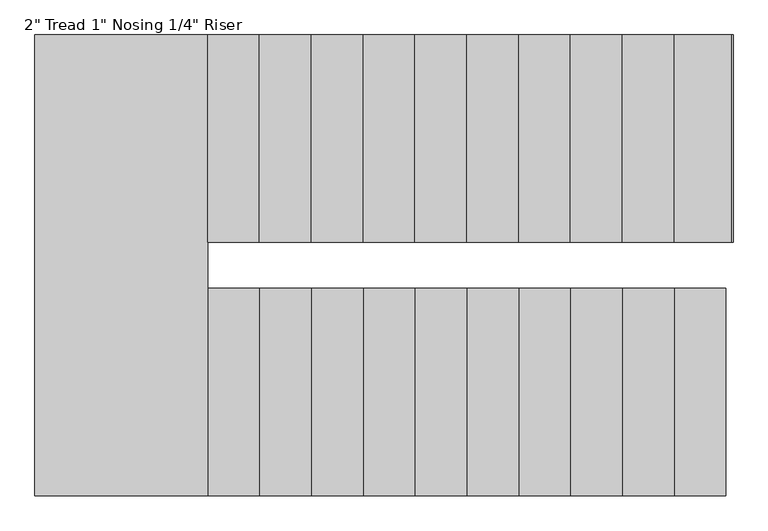
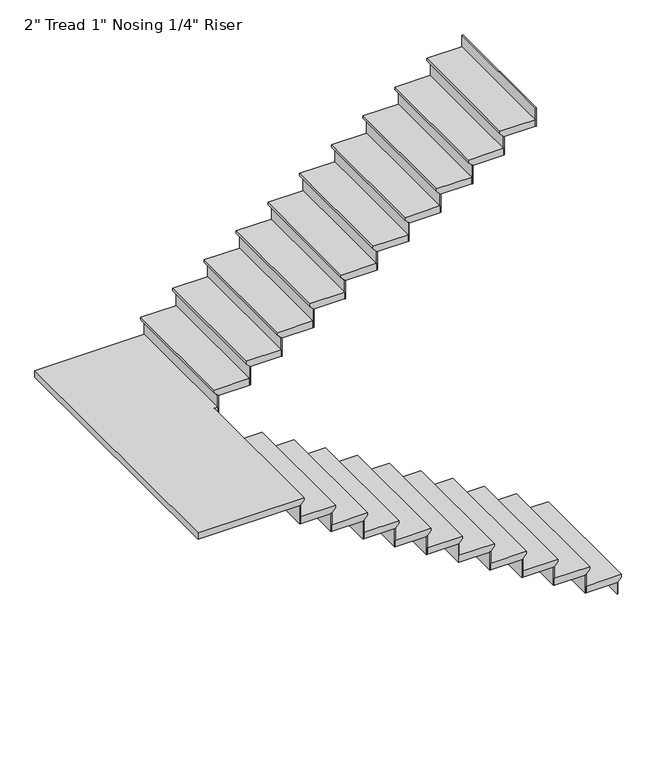
"""IFC4 building model written with IfcOpenShell, lengths in millimetres: stair flight geometry."""

from ifc_helpers import new_model, si_unit, origin, place, context, project, spatial, faceted_brep, source, transform, mapped, element, save


def stair_flight_0d4d62c4(model_context):
    return source(origin(), model_context, "Body", "Brep", [
        faceted_brep([(-2080.8410855, 332.1803617, 16121.4954545), (-2080.8410855, 332.1803617, 16140.5454545), (-2080.8410855, -582.2196383, 16140.5454545), (-2080.8410855, -582.2196383, 16121.4954545), (-2106.2410855, 332.1803617, 16096.0954545), (-2106.2410855, -582.2196383, 16096.0954545), (-2334.8410855, 332.1803617, 16140.5454545), (-2334.8410855, -582.2196383, 16140.5454545), (-2106.2410855, -582.2196383, 16089.7454545), (-2334.8410855, -582.2196383, 16089.7454545), (-2334.8410855, 332.1803617, 16089.7454545), (-2106.2410855, 332.1803617, 16089.7454545)], [[[0, 1, 2, 3]], [[4, 0, 3, 5]], [[2, 1, 6, 7]], [[8, 9, 10, 11]], [[2, 7, 9, 8, 5, 3]], [[8, 11, 4, 5]], [[6, 1, 0, 4, 11, 10]], [[7, 6, 10, 9]]]),
        faceted_brep([(-2106.2410855, 332.1803617, 16089.7454545), (-2106.2410855, 332.1803617, 16002.0), (-2112.5910855, 332.1803617, 16002.0), (-2112.5910855, 332.1803617, 16089.7454545), (-2106.2410855, -582.2196383, 16089.7454545), (-2112.5910855, -582.2196383, 16089.7454545), (-2112.5910855, -582.2196383, 16002.0), (-2106.2410855, -582.2196383, 16002.0)], [[[0, 1, 2, 3]], [[4, 5, 6, 7]], [[1, 0, 4, 7]], [[2, 1, 7, 6]], [[3, 2, 6, 5]], [[0, 3, 5, 4]]]),
        faceted_brep([(-2334.8410855, 332.1803617, 16228.2909091), (-2334.8410855, 332.1803617, 16089.7454545), (-2341.1910855, 332.1803617, 16089.7454545), (-2341.1910855, 332.1803617, 16228.2909091), (-2334.8410855, -582.2196383, 16228.2909091), (-2341.1910855, -582.2196383, 16228.2909091), (-2341.1910855, -582.2196383, 16089.7454545), (-2334.8410855, -582.2196383, 16089.7454545)], [[[0, 1, 2, 3]], [[4, 5, 6, 7]], [[1, 0, 4, 7]], [[2, 1, 7, 6]], [[3, 2, 6, 5]], [[0, 3, 5, 4]]]),
        faceted_brep([(-2309.4410855, -582.2196383, 16279.0909091), (-2309.4410855, 332.1803617, 16279.0909091), (-2563.4410855, 332.1803617, 16279.0909091), (-2563.4410855, -582.2196383, 16279.0909091), (-2334.8410855, -582.2196383, 16228.2909091), (-2563.4410855, -582.2196383, 16228.2909091), (-2563.4410855, 332.1803617, 16228.2909091), (-2334.8410855, 332.1803617, 16228.2909091), (-2334.8410855, -582.2196383, 16234.6409091), (-2309.4410855, -582.2196383, 16260.0409091), (-2334.8410855, 332.1803617, 16234.6409091), (-2309.4410855, 332.1803617, 16260.0409091)], [[[0, 1, 2, 3]], [[4, 5, 6, 7]], [[0, 3, 5, 4, 8, 9]], [[4, 7, 10, 8]], [[2, 1, 11, 10, 7, 6]], [[3, 2, 6, 5]], [[11, 1, 0, 9]], [[10, 11, 9, 8]]]),
        faceted_brep([(-2563.4410855, 332.1803617, 16366.8363636), (-2563.4410855, 332.1803617, 16228.2909091), (-2569.7910855, 332.1803617, 16228.2909091), (-2569.7910855, 332.1803617, 16366.8363636), (-2563.4410855, -582.2196383, 16366.8363636), (-2569.7910855, -582.2196383, 16366.8363636), (-2569.7910855, -582.2196383, 16228.2909091), (-2563.4410855, -582.2196383, 16228.2909091)], [[[0, 1, 2, 3]], [[4, 5, 6, 7]], [[1, 0, 4, 7]], [[2, 1, 7, 6]], [[3, 2, 6, 5]], [[0, 3, 5, 4]]]),
        faceted_brep([(-2538.0410855, -582.2196383, 16417.6363636), (-2538.0410855, 332.1803617, 16417.6363636), (-2792.0410855, 332.1803617, 16417.6363636), (-2792.0410855, -582.2196383, 16417.6363636), (-2563.4410855, -582.2196383, 16366.8363636), (-2792.0410855, -582.2196383, 16366.8363636), (-2792.0410855, 332.1803617, 16366.8363636), (-2563.4410855, 332.1803617, 16366.8363636), (-2563.4410855, -582.2196383, 16373.1863636), (-2538.0410855, -582.2196383, 16398.5863636), (-2563.4410855, 332.1803617, 16373.1863636), (-2538.0410855, 332.1803617, 16398.5863636)], [[[0, 1, 2, 3]], [[4, 5, 6, 7]], [[0, 3, 5, 4, 8, 9]], [[4, 7, 10, 8]], [[2, 1, 11, 10, 7, 6]], [[3, 2, 6, 5]], [[11, 1, 0, 9]], [[10, 11, 9, 8]]]),
        faceted_brep([(-2792.0410855, 332.1803617, 16505.3818182), (-2792.0410855, 332.1803617, 16366.8363636), (-2798.3910855, 332.1803617, 16366.8363636), (-2798.3910855, 332.1803617, 16505.3818182), (-2792.0410855, -582.2196383, 16505.3818182), (-2798.3910855, -582.2196383, 16505.3818182), (-2798.3910855, -582.2196383, 16366.8363636), (-2792.0410855, -582.2196383, 16366.8363636)], [[[0, 1, 2, 3]], [[4, 5, 6, 7]], [[1, 0, 4, 7]], [[2, 1, 7, 6]], [[3, 2, 6, 5]], [[0, 3, 5, 4]]]),
        faceted_brep([(-2766.6410855, -582.2196383, 16556.1818182), (-2766.6410855, 332.1803617, 16556.1818182), (-3020.6410855, 332.1803617, 16556.1818182), (-3020.6410855, -582.2196383, 16556.1818182), (-2792.0410855, -582.2196383, 16505.3818182), (-3020.6410855, -582.2196383, 16505.3818182), (-3020.6410855, 332.1803617, 16505.3818182), (-2792.0410855, 332.1803617, 16505.3818182), (-2792.0410855, -582.2196383, 16511.7318182), (-2766.6410855, -582.2196383, 16537.1318182), (-2792.0410855, 332.1803617, 16511.7318182), (-2766.6410855, 332.1803617, 16537.1318182)], [[[0, 1, 2, 3]], [[4, 5, 6, 7]], [[0, 3, 5, 4, 8, 9]], [[4, 7, 10, 8]], [[2, 1, 11, 10, 7, 6]], [[3, 2, 6, 5]], [[11, 1, 0, 9]], [[10, 11, 9, 8]]]),
        faceted_brep([(-3020.6410855, 332.1803617, 16643.9272727), (-3020.6410855, 332.1803617, 16505.3818182), (-3026.9910855, 332.1803617, 16505.3818182), (-3026.9910855, 332.1803617, 16643.9272727), (-3020.6410855, -582.2196383, 16643.9272727), (-3026.9910855, -582.2196383, 16643.9272727), (-3026.9910855, -582.2196383, 16505.3818182), (-3020.6410855, -582.2196383, 16505.3818182)], [[[0, 1, 2, 3]], [[4, 5, 6, 7]], [[1, 0, 4, 7]], [[2, 1, 7, 6]], [[3, 2, 6, 5]], [[0, 3, 5, 4]]]),
        faceted_brep([(-2995.2410855, -582.2196383, 16694.7272727), (-2995.2410855, 332.1803617, 16694.7272727), (-3249.2410855, 332.1803617, 16694.7272727), (-3249.2410855, -582.2196383, 16694.7272727), (-3020.6410855, -582.2196383, 16643.9272727), (-3249.2410855, -582.2196383, 16643.9272727), (-3249.2410855, 332.1803617, 16643.9272727), (-3020.6410855, 332.1803617, 16643.9272727), (-3020.6410855, -582.2196383, 16650.2772727), (-2995.2410855, -582.2196383, 16675.6772727), (-3020.6410855, 332.1803617, 16650.2772727), (-2995.2410855, 332.1803617, 16675.6772727)], [[[0, 1, 2, 3]], [[4, 5, 6, 7]], [[0, 3, 5, 4, 8, 9]], [[4, 7, 10, 8]], [[2, 1, 11, 10, 7, 6]], [[3, 2, 6, 5]], [[11, 1, 0, 9]], [[10, 11, 9, 8]]]),
        faceted_brep([(-3249.2410855, 332.1803617, 16782.4727273), (-3249.2410855, 332.1803617, 16643.9272727), (-3255.5910855, 332.1803617, 16643.9272727), (-3255.5910855, 332.1803617, 16782.4727273), (-3249.2410855, -582.2196383, 16782.4727273), (-3255.5910855, -582.2196383, 16782.4727273), (-3255.5910855, -582.2196383, 16643.9272727), (-3249.2410855, -582.2196383, 16643.9272727)], [[[0, 1, 2, 3]], [[4, 5, 6, 7]], [[1, 0, 4, 7]], [[2, 1, 7, 6]], [[3, 2, 6, 5]], [[0, 3, 5, 4]]]),
        faceted_brep([(-3223.8410855, -582.2196383, 16833.2727273), (-3223.8410855, 332.1803617, 16833.2727273), (-3477.8410855, 332.1803617, 16833.2727273), (-3477.8410855, -582.2196383, 16833.2727273), (-3249.2410855, -582.2196383, 16782.4727273), (-3477.8410855, -582.2196383, 16782.4727273), (-3477.8410855, 332.1803617, 16782.4727273), (-3249.2410855, 332.1803617, 16782.4727273), (-3249.2410855, -582.2196383, 16788.8227273), (-3223.8410855, -582.2196383, 16814.2227273), (-3249.2410855, 332.1803617, 16788.8227273), (-3223.8410855, 332.1803617, 16814.2227273)], [[[0, 1, 2, 3]], [[4, 5, 6, 7]], [[0, 3, 5, 4, 8, 9]], [[4, 7, 10, 8]], [[2, 1, 11, 10, 7, 6]], [[3, 2, 6, 5]], [[11, 1, 0, 9]], [[10, 11, 9, 8]]]),
        faceted_brep([(-3477.8410855, 332.1803617, 16921.0181818), (-3477.8410855, 332.1803617, 16782.4727273), (-3484.1910855, 332.1803617, 16782.4727273), (-3484.1910855, 332.1803617, 16921.0181818), (-3477.8410855, -582.2196383, 16921.0181818), (-3484.1910855, -582.2196383, 16921.0181818), (-3484.1910855, -582.2196383, 16782.4727273), (-3477.8410855, -582.2196383, 16782.4727273)], [[[0, 1, 2, 3]], [[4, 5, 6, 7]], [[1, 0, 4, 7]], [[2, 1, 7, 6]], [[3, 2, 6, 5]], [[0, 3, 5, 4]]]),
        faceted_brep([(-3452.4410855, -582.2196383, 16971.8181818), (-3452.4410855, 332.1803617, 16971.8181818), (-3706.4410855, 332.1803617, 16971.8181818), (-3706.4410855, -582.2196383, 16971.8181818), (-3477.8410855, -582.2196383, 16921.0181818), (-3706.4410855, -582.2196383, 16921.0181818), (-3706.4410855, 332.1803617, 16921.0181818), (-3477.8410855, 332.1803617, 16921.0181818), (-3477.8410855, -582.2196383, 16927.3681818), (-3452.4410855, -582.2196383, 16952.7681818), (-3477.8410855, 332.1803617, 16927.3681818), (-3452.4410855, 332.1803617, 16952.7681818)], [[[0, 1, 2, 3]], [[4, 5, 6, 7]], [[0, 3, 5, 4, 8, 9]], [[4, 7, 10, 8]], [[2, 1, 11, 10, 7, 6]], [[3, 2, 6, 5]], [[11, 1, 0, 9]], [[10, 11, 9, 8]]]),
        faceted_brep([(-3706.4410855, 332.1803617, 17059.5636364), (-3706.4410855, 332.1803617, 16921.0181818), (-3712.7910855, 332.1803617, 16921.0181818), (-3712.7910855, 332.1803617, 17059.5636364), (-3706.4410855, -582.2196383, 17059.5636364), (-3712.7910855, -582.2196383, 17059.5636364), (-3712.7910855, -582.2196383, 16921.0181818), (-3706.4410855, -582.2196383, 16921.0181818)], [[[0, 1, 2, 3]], [[4, 5, 6, 7]], [[1, 0, 4, 7]], [[2, 1, 7, 6]], [[3, 2, 6, 5]], [[0, 3, 5, 4]]]),
        faceted_brep([(-3681.0410855, -582.2196383, 17110.3636364), (-3681.0410855, 332.1803617, 17110.3636364), (-3935.0410855, 332.1803617, 17110.3636364), (-3935.0410855, -582.2196383, 17110.3636364), (-3706.4410855, -582.2196383, 17059.5636364), (-3935.0410855, -582.2196383, 17059.5636364), (-3935.0410855, 332.1803617, 17059.5636364), (-3706.4410855, 332.1803617, 17059.5636364), (-3706.4410855, -582.2196383, 17065.9136364), (-3681.0410855, -582.2196383, 17091.3136364), (-3706.4410855, 332.1803617, 17065.9136364), (-3681.0410855, 332.1803617, 17091.3136364)], [[[0, 1, 2, 3]], [[4, 5, 6, 7]], [[0, 3, 5, 4, 8, 9]], [[4, 7, 10, 8]], [[2, 1, 11, 10, 7, 6]], [[3, 2, 6, 5]], [[11, 1, 0, 9]], [[10, 11, 9, 8]]]),
        faceted_brep([(-3935.0410855, 332.1803617, 17198.1090909), (-3935.0410855, 332.1803617, 17059.5636364), (-3941.3910855, 332.1803617, 17059.5636364), (-3941.3910855, 332.1803617, 17198.1090909), (-3935.0410855, -582.2196383, 17198.1090909), (-3941.3910855, -582.2196383, 17198.1090909), (-3941.3910855, -582.2196383, 17059.5636364), (-3935.0410855, -582.2196383, 17059.5636364)], [[[0, 1, 2, 3]], [[4, 5, 6, 7]], [[1, 0, 4, 7]], [[2, 1, 7, 6]], [[3, 2, 6, 5]], [[0, 3, 5, 4]]]),
        faceted_brep([(-3909.6410855, -582.2196383, 17248.9090909), (-3909.6410855, 332.1803617, 17248.9090909), (-4163.6410855, 332.1803617, 17248.9090909), (-4163.6410855, -582.2196383, 17248.9090909), (-3935.0410855, -582.2196383, 17198.1090909), (-4163.6410855, -582.2196383, 17198.1090909), (-4163.6410855, 332.1803617, 17198.1090909), (-3935.0410855, 332.1803617, 17198.1090909), (-3935.0410855, -582.2196383, 17204.4590909), (-3909.6410855, -582.2196383, 17229.8590909), (-3935.0410855, 332.1803617, 17204.4590909), (-3909.6410855, 332.1803617, 17229.8590909)], [[[0, 1, 2, 3]], [[4, 5, 6, 7]], [[0, 3, 5, 4, 8, 9]], [[4, 7, 10, 8]], [[2, 1, 11, 10, 7, 6]], [[3, 2, 6, 5]], [[11, 1, 0, 9]], [[10, 11, 9, 8]]]),
        faceted_brep([(-4163.6410855, 332.1803617, 17336.6545455), (-4163.6410855, 332.1803617, 17198.1090909), (-4169.9910855, 332.1803617, 17198.1090909), (-4169.9910855, 332.1803617, 17336.6545455), (-4163.6410855, -582.2196383, 17336.6545455), (-4169.9910855, -582.2196383, 17336.6545455), (-4169.9910855, -582.2196383, 17198.1090909), (-4163.6410855, -582.2196383, 17198.1090909)], [[[0, 1, 2, 3]], [[4, 5, 6, 7]], [[1, 0, 4, 7]], [[2, 1, 7, 6]], [[3, 2, 6, 5]], [[0, 3, 5, 4]]]),
        faceted_brep([(-4138.2410855, -582.2196383, 17387.4545455), (-4138.2410855, 332.1803617, 17387.4545455), (-4392.2410855, 332.1803617, 17387.4545455), (-4392.2410855, -582.2196383, 17387.4545455), (-4163.6410855, -582.2196383, 17336.6545455), (-4392.2410855, -582.2196383, 17336.6545455), (-4392.2410855, 332.1803617, 17336.6545455), (-4163.6410855, 332.1803617, 17336.6545455), (-4163.6410855, -582.2196383, 17343.0045455), (-4138.2410855, -582.2196383, 17368.4045455), (-4163.6410855, 332.1803617, 17343.0045455), (-4138.2410855, 332.1803617, 17368.4045455)], [[[0, 1, 2, 3]], [[4, 5, 6, 7]], [[0, 3, 5, 4, 8, 9]], [[4, 7, 10, 8]], [[2, 1, 11, 10, 7, 6]], [[3, 2, 6, 5]], [[11, 1, 0, 9]], [[10, 11, 9, 8]]]),
        faceted_brep([(-4392.2410855, 332.1803617, 17475.2), (-4392.2410855, 332.1803617, 17336.6545455), (-4398.5910855, 332.1803617, 17336.6545455), (-4398.5910855, 332.1803617, 17475.2), (-4392.2410855, -582.2196383, 17475.2), (-4398.5910855, -582.2196383, 17475.2), (-4398.5910855, -582.2196383, 17336.6545455), (-4392.2410855, -582.2196383, 17336.6545455)], [[[0, 1, 2, 3]], [[4, 5, 6, 7]], [[1, 0, 4, 7]], [[2, 1, 7, 6]], [[3, 2, 6, 5]], [[0, 3, 5, 4]]]),
        faceted_brep([(-4341.4410855, 1449.7803617, 17526.0), (-5128.8410855, 1449.7803617, 17526.0), (-5128.8410855, -582.2196383, 17526.0), (-4366.8410855, -582.2196383, 17526.0), (-4366.8410855, 535.3803617, 17526.0), (-4341.4410855, 535.3803617, 17526.0), (-5128.8410855, 1449.7803617, 17475.2), (-4341.4410855, 1449.7803617, 17475.2), (-4341.4410855, 535.3803617, 17475.2), (-4366.8410855, 535.3803617, 17475.2), (-4366.8410855, 332.1803617, 17475.2), (-4392.2410855, 332.1803617, 17475.2), (-4392.2410855, -582.2196383, 17475.2), (-5128.8410855, -582.2196383, 17475.2), (-4392.2410855, -582.2196383, 17481.55), (-4366.8410855, -582.2196383, 17506.95), (-4392.2410855, 332.1803617, 17481.55), (-4366.8410855, 332.1803617, 17506.95)], [[[0, 1, 2, 3, 4, 5]], [[6, 7, 8, 9, 10, 11, 12, 13]], [[1, 0, 7, 6]], [[2, 1, 6, 13]], [[3, 2, 13, 12, 14, 15]], [[12, 11, 16, 14]], [[11, 10, 17, 16]], [[4, 3, 15, 17, 10, 9]], [[5, 4, 9, 8]], [[0, 5, 8, 7]], [[15, 14, 16, 17]]]),
        faceted_brep([(-4341.4410855, 535.3803617, 17613.7454545), (-4341.4410855, 535.3803617, 17475.2), (-4335.0910855, 535.3803617, 17475.2), (-4335.0910855, 535.3803617, 17613.7454545), (-4341.4410855, 1449.7803617, 17613.7454545), (-4335.0910855, 1449.7803617, 17613.7454545), (-4335.0910855, 1449.7803617, 17475.2), (-4341.4410855, 1449.7803617, 17475.2)], [[[0, 1, 2, 3]], [[4, 5, 6, 7]], [[1, 0, 4, 7]], [[2, 1, 7, 6]], [[3, 2, 6, 5]], [[0, 3, 5, 4]]]),
        faceted_brep([(-4366.8410855, 1449.7803617, 17664.5454545), (-4366.8410855, 535.3803617, 17664.5454545), (-4112.8410855, 535.3803617, 17664.5454545), (-4112.8410855, 1449.7803617, 17664.5454545), (-4341.4410855, 1449.7803617, 17613.7454545), (-4112.8410855, 1449.7803617, 17613.7454545), (-4112.8410855, 535.3803617, 17613.7454545), (-4341.4410855, 535.3803617, 17613.7454545), (-4341.4410855, 1449.7803617, 17620.0954545), (-4366.8410855, 1449.7803617, 17645.4954545), (-4341.4410855, 535.3803617, 17620.0954545), (-4366.8410855, 535.3803617, 17645.4954545)], [[[0, 1, 2, 3]], [[4, 5, 6, 7]], [[0, 3, 5, 4, 8, 9]], [[4, 7, 10, 8]], [[2, 1, 11, 10, 7, 6]], [[3, 2, 6, 5]], [[11, 1, 0, 9]], [[10, 11, 9, 8]]]),
        faceted_brep([(-4112.8410855, 535.3803617, 17752.2909091), (-4112.8410855, 535.3803617, 17613.7454545), (-4106.4910855, 535.3803617, 17613.7454545), (-4106.4910855, 535.3803617, 17752.2909091), (-4112.8410855, 1449.7803617, 17752.2909091), (-4106.4910855, 1449.7803617, 17752.2909091), (-4106.4910855, 1449.7803617, 17613.7454545), (-4112.8410855, 1449.7803617, 17613.7454545)], [[[0, 1, 2, 3]], [[4, 5, 6, 7]], [[1, 0, 4, 7]], [[2, 1, 7, 6]], [[3, 2, 6, 5]], [[0, 3, 5, 4]]]),
        faceted_brep([(-4138.2410855, 1449.7803617, 17803.0909091), (-4138.2410855, 535.3803617, 17803.0909091), (-3884.2410855, 535.3803617, 17803.0909091), (-3884.2410855, 1449.7803617, 17803.0909091), (-4112.8410855, 1449.7803617, 17752.2909091), (-3884.2410855, 1449.7803617, 17752.2909091), (-3884.2410855, 535.3803617, 17752.2909091), (-4112.8410855, 535.3803617, 17752.2909091), (-4112.8410855, 1449.7803617, 17758.6409091), (-4138.2410855, 1449.7803617, 17784.0409091), (-4112.8410855, 535.3803617, 17758.6409091), (-4138.2410855, 535.3803617, 17784.0409091)], [[[0, 1, 2, 3]], [[4, 5, 6, 7]], [[0, 3, 5, 4, 8, 9]], [[4, 7, 10, 8]], [[2, 1, 11, 10, 7, 6]], [[3, 2, 6, 5]], [[11, 1, 0, 9]], [[10, 11, 9, 8]]]),
        faceted_brep([(-3884.2410855, 535.3803617, 17890.8363636), (-3884.2410855, 535.3803617, 17752.2909091), (-3877.8910855, 535.3803617, 17752.2909091), (-3877.8910855, 535.3803617, 17890.8363636), (-3884.2410855, 1449.7803617, 17890.8363636), (-3877.8910855, 1449.7803617, 17890.8363636), (-3877.8910855, 1449.7803617, 17752.2909091), (-3884.2410855, 1449.7803617, 17752.2909091)], [[[0, 1, 2, 3]], [[4, 5, 6, 7]], [[1, 0, 4, 7]], [[2, 1, 7, 6]], [[3, 2, 6, 5]], [[0, 3, 5, 4]]]),
        faceted_brep([(-3909.6410855, 1449.7803617, 17941.6363636), (-3909.6410855, 535.3803617, 17941.6363636), (-3655.6410855, 535.3803617, 17941.6363636), (-3655.6410855, 1449.7803617, 17941.6363636), (-3884.2410855, 1449.7803617, 17890.8363636), (-3655.6410855, 1449.7803617, 17890.8363636), (-3655.6410855, 535.3803617, 17890.8363636), (-3884.2410855, 535.3803617, 17890.8363636), (-3884.2410855, 1449.7803617, 17897.1863636), (-3909.6410855, 1449.7803617, 17922.5863636), (-3884.2410855, 535.3803617, 17897.1863636), (-3909.6410855, 535.3803617, 17922.5863636)], [[[0, 1, 2, 3]], [[4, 5, 6, 7]], [[0, 3, 5, 4, 8, 9]], [[4, 7, 10, 8]], [[2, 1, 11, 10, 7, 6]], [[3, 2, 6, 5]], [[11, 1, 0, 9]], [[10, 11, 9, 8]]]),
        faceted_brep([(-3655.6410855, 535.3803617, 18029.3818182), (-3655.6410855, 535.3803617, 17890.8363636), (-3649.2910855, 535.3803617, 17890.8363636), (-3649.2910855, 535.3803617, 18029.3818182), (-3655.6410855, 1449.7803617, 18029.3818182), (-3649.2910855, 1449.7803617, 18029.3818182), (-3649.2910855, 1449.7803617, 17890.8363636), (-3655.6410855, 1449.7803617, 17890.8363636)], [[[0, 1, 2, 3]], [[4, 5, 6, 7]], [[1, 0, 4, 7]], [[2, 1, 7, 6]], [[3, 2, 6, 5]], [[0, 3, 5, 4]]]),
        faceted_brep([(-3681.0410855, 1449.7803617, 18080.1818182), (-3681.0410855, 535.3803617, 18080.1818182), (-3427.0410855, 535.3803617, 18080.1818182), (-3427.0410855, 1449.7803617, 18080.1818182), (-3655.6410855, 1449.7803617, 18029.3818182), (-3427.0410855, 1449.7803617, 18029.3818182), (-3427.0410855, 535.3803617, 18029.3818182), (-3655.6410855, 535.3803617, 18029.3818182), (-3655.6410855, 1449.7803617, 18035.7318182), (-3681.0410855, 1449.7803617, 18061.1318182), (-3655.6410855, 535.3803617, 18035.7318182), (-3681.0410855, 535.3803617, 18061.1318182)], [[[0, 1, 2, 3]], [[4, 5, 6, 7]], [[0, 3, 5, 4, 8, 9]], [[4, 7, 10, 8]], [[2, 1, 11, 10, 7, 6]], [[3, 2, 6, 5]], [[11, 1, 0, 9]], [[10, 11, 9, 8]]]),
        faceted_brep([(-3427.0410855, 535.3803617, 18167.9272727), (-3427.0410855, 535.3803617, 18029.3818182), (-3420.6910855, 535.3803617, 18029.3818182), (-3420.6910855, 535.3803617, 18167.9272727), (-3427.0410855, 1449.7803617, 18167.9272727), (-3420.6910855, 1449.7803617, 18167.9272727), (-3420.6910855, 1449.7803617, 18029.3818182), (-3427.0410855, 1449.7803617, 18029.3818182)], [[[0, 1, 2, 3]], [[4, 5, 6, 7]], [[1, 0, 4, 7]], [[2, 1, 7, 6]], [[3, 2, 6, 5]], [[0, 3, 5, 4]]]),
        faceted_brep([(-3452.4410855, 1449.7803617, 18218.7272727), (-3452.4410855, 535.3803617, 18218.7272727), (-3198.4410855, 535.3803617, 18218.7272727), (-3198.4410855, 1449.7803617, 18218.7272727), (-3427.0410855, 1449.7803617, 18167.9272727), (-3198.4410855, 1449.7803617, 18167.9272727), (-3198.4410855, 535.3803617, 18167.9272727), (-3427.0410855, 535.3803617, 18167.9272727), (-3427.0410855, 1449.7803617, 18174.2772727), (-3452.4410855, 1449.7803617, 18199.6772727), (-3427.0410855, 535.3803617, 18174.2772727), (-3452.4410855, 535.3803617, 18199.6772727)], [[[0, 1, 2, 3]], [[4, 5, 6, 7]], [[0, 3, 5, 4, 8, 9]], [[4, 7, 10, 8]], [[2, 1, 11, 10, 7, 6]], [[3, 2, 6, 5]], [[11, 1, 0, 9]], [[10, 11, 9, 8]]]),
        faceted_brep([(-3198.4410855, 535.3803617, 18306.4727273), (-3198.4410855, 535.3803617, 18167.9272727), (-3192.0910855, 535.3803617, 18167.9272727), (-3192.0910855, 535.3803617, 18306.4727273), (-3198.4410855, 1449.7803617, 18306.4727273), (-3192.0910855, 1449.7803617, 18306.4727273), (-3192.0910855, 1449.7803617, 18167.9272727), (-3198.4410855, 1449.7803617, 18167.9272727)], [[[0, 1, 2, 3]], [[4, 5, 6, 7]], [[1, 0, 4, 7]], [[2, 1, 7, 6]], [[3, 2, 6, 5]], [[0, 3, 5, 4]]]),
        faceted_brep([(-3223.8410855, 1449.7803617, 18357.2727273), (-3223.8410855, 535.3803617, 18357.2727273), (-2969.8410855, 535.3803617, 18357.2727273), (-2969.8410855, 1449.7803617, 18357.2727273), (-3198.4410855, 1449.7803617, 18306.4727273), (-2969.8410855, 1449.7803617, 18306.4727273), (-2969.8410855, 535.3803617, 18306.4727273), (-3198.4410855, 535.3803617, 18306.4727273), (-3198.4410855, 1449.7803617, 18312.8227273), (-3223.8410855, 1449.7803617, 18338.2227273), (-3198.4410855, 535.3803617, 18312.8227273), (-3223.8410855, 535.3803617, 18338.2227273)], [[[0, 1, 2, 3]], [[4, 5, 6, 7]], [[0, 3, 5, 4, 8, 9]], [[4, 7, 10, 8]], [[2, 1, 11, 10, 7, 6]], [[3, 2, 6, 5]], [[11, 1, 0, 9]], [[10, 11, 9, 8]]]),
        faceted_brep([(-2969.8410855, 535.3803617, 18445.0181818), (-2969.8410855, 535.3803617, 18306.4727273), (-2963.4910855, 535.3803617, 18306.4727273), (-2963.4910855, 535.3803617, 18445.0181818), (-2969.8410855, 1449.7803617, 18445.0181818), (-2963.4910855, 1449.7803617, 18445.0181818), (-2963.4910855, 1449.7803617, 18306.4727273), (-2969.8410855, 1449.7803617, 18306.4727273)], [[[0, 1, 2, 3]], [[4, 5, 6, 7]], [[1, 0, 4, 7]], [[2, 1, 7, 6]], [[3, 2, 6, 5]], [[0, 3, 5, 4]]]),
        faceted_brep([(-2995.2410855, 1449.7803617, 18495.8181818), (-2995.2410855, 535.3803617, 18495.8181818), (-2741.2410855, 535.3803617, 18495.8181818), (-2741.2410855, 1449.7803617, 18495.8181818), (-2969.8410855, 1449.7803617, 18445.0181818), (-2741.2410855, 1449.7803617, 18445.0181818), (-2741.2410855, 535.3803617, 18445.0181818), (-2969.8410855, 535.3803617, 18445.0181818), (-2969.8410855, 1449.7803617, 18451.3681818), (-2995.2410855, 1449.7803617, 18476.7681818), (-2969.8410855, 535.3803617, 18451.3681818), (-2995.2410855, 535.3803617, 18476.7681818)], [[[0, 1, 2, 3]], [[4, 5, 6, 7]], [[0, 3, 5, 4, 8, 9]], [[4, 7, 10, 8]], [[2, 1, 11, 10, 7, 6]], [[3, 2, 6, 5]], [[11, 1, 0, 9]], [[10, 11, 9, 8]]]),
        faceted_brep([(-2741.2410855, 535.3803617, 18583.5636364), (-2741.2410855, 535.3803617, 18445.0181818), (-2734.8910855, 535.3803617, 18445.0181818), (-2734.8910855, 535.3803617, 18583.5636364), (-2741.2410855, 1449.7803617, 18583.5636364), (-2734.8910855, 1449.7803617, 18583.5636364), (-2734.8910855, 1449.7803617, 18445.0181818), (-2741.2410855, 1449.7803617, 18445.0181818)], [[[0, 1, 2, 3]], [[4, 5, 6, 7]], [[1, 0, 4, 7]], [[2, 1, 7, 6]], [[3, 2, 6, 5]], [[0, 3, 5, 4]]]),
        faceted_brep([(-2766.6410855, 1449.7803617, 18634.3636364), (-2766.6410855, 535.3803617, 18634.3636364), (-2512.6410855, 535.3803617, 18634.3636364), (-2512.6410855, 1449.7803617, 18634.3636364), (-2741.2410855, 1449.7803617, 18583.5636364), (-2512.6410855, 1449.7803617, 18583.5636364), (-2512.6410855, 535.3803617, 18583.5636364), (-2741.2410855, 535.3803617, 18583.5636364), (-2741.2410855, 1449.7803617, 18589.9136364), (-2766.6410855, 1449.7803617, 18615.3136364), (-2741.2410855, 535.3803617, 18589.9136364), (-2766.6410855, 535.3803617, 18615.3136364)], [[[0, 1, 2, 3]], [[4, 5, 6, 7]], [[0, 3, 5, 4, 8, 9]], [[4, 7, 10, 8]], [[2, 1, 11, 10, 7, 6]], [[3, 2, 6, 5]], [[11, 1, 0, 9]], [[10, 11, 9, 8]]]),
        faceted_brep([(-2512.6410855, 535.3803617, 18722.1090909), (-2512.6410855, 535.3803617, 18583.5636364), (-2506.2910855, 535.3803617, 18583.5636364), (-2506.2910855, 535.3803617, 18722.1090909), (-2512.6410855, 1449.7803617, 18722.1090909), (-2506.2910855, 1449.7803617, 18722.1090909), (-2506.2910855, 1449.7803617, 18583.5636364), (-2512.6410855, 1449.7803617, 18583.5636364)], [[[0, 1, 2, 3]], [[4, 5, 6, 7]], [[1, 0, 4, 7]], [[2, 1, 7, 6]], [[3, 2, 6, 5]], [[0, 3, 5, 4]]]),
        faceted_brep([(-2538.0410855, 1449.7803617, 18772.9090909), (-2538.0410855, 535.3803617, 18772.9090909), (-2284.0410855, 535.3803617, 18772.9090909), (-2284.0410855, 1449.7803617, 18772.9090909), (-2512.6410855, 1449.7803617, 18722.1090909), (-2284.0410855, 1449.7803617, 18722.1090909), (-2284.0410855, 535.3803617, 18722.1090909), (-2512.6410855, 535.3803617, 18722.1090909), (-2512.6410855, 1449.7803617, 18728.4590909), (-2538.0410855, 1449.7803617, 18753.8590909), (-2512.6410855, 535.3803617, 18728.4590909), (-2538.0410855, 535.3803617, 18753.8590909)], [[[0, 1, 2, 3]], [[4, 5, 6, 7]], [[0, 3, 5, 4, 8, 9]], [[4, 7, 10, 8]], [[2, 1, 11, 10, 7, 6]], [[3, 2, 6, 5]], [[11, 1, 0, 9]], [[10, 11, 9, 8]]]),
        faceted_brep([(-2284.0410855, 535.3803617, 18860.6545455), (-2284.0410855, 535.3803617, 18722.1090909), (-2277.6910855, 535.3803617, 18722.1090909), (-2277.6910855, 535.3803617, 18860.6545455), (-2284.0410855, 1449.7803617, 18860.6545455), (-2277.6910855, 1449.7803617, 18860.6545455), (-2277.6910855, 1449.7803617, 18722.1090909), (-2284.0410855, 1449.7803617, 18722.1090909)], [[[0, 1, 2, 3]], [[4, 5, 6, 7]], [[1, 0, 4, 7]], [[2, 1, 7, 6]], [[3, 2, 6, 5]], [[0, 3, 5, 4]]]),
        faceted_brep([(-2055.4410855, 535.3803617, 18999.2), (-2055.4410855, 535.3803617, 18860.6545455), (-2049.0910855, 535.3803617, 18860.6545455), (-2049.0910855, 535.3803617, 18999.2), (-2055.4410855, 1449.7803617, 18999.2), (-2049.0910855, 1449.7803617, 18999.2), (-2049.0910855, 1449.7803617, 18860.6545455), (-2055.4410855, 1449.7803617, 18860.6545455)], [[[0, 1, 2, 3]], [[4, 5, 6, 7]], [[1, 0, 4, 7]], [[2, 1, 7, 6]], [[3, 2, 6, 5]], [[0, 3, 5, 4]]]),
        faceted_brep([(-2309.4410855, 1449.7803617, 18911.4545455), (-2309.4410855, 535.3803617, 18911.4545455), (-2055.4410855, 535.3803617, 18911.4545455), (-2055.4410855, 1449.7803617, 18911.4545455), (-2284.0410855, 1449.7803617, 18860.6545455), (-2055.4410855, 1449.7803617, 18860.6545455), (-2055.4410855, 535.3803617, 18860.6545455), (-2284.0410855, 535.3803617, 18860.6545455), (-2284.0410855, 1449.7803617, 18867.0045455), (-2309.4410855, 1449.7803617, 18892.4045455), (-2284.0410855, 535.3803617, 18867.0045455), (-2309.4410855, 535.3803617, 18892.4045455)], [[[0, 1, 2, 3]], [[4, 5, 6, 7]], [[0, 3, 5, 4, 8, 9]], [[4, 7, 10, 8]], [[2, 1, 11, 10, 7, 6]], [[3, 2, 6, 5]], [[11, 1, 0, 9]], [[10, 11, 9, 8]]]),
    ])


if __name__ == "__main__":
    model = new_model("IFC4")
    model_context = context("Model", 3, world=origin())
    ifc_project = project(units=[si_unit("LENGTHUNIT", "METRE", prefix="MILLI")], contexts=[model_context])
    site = spatial("IfcSite", under=ifc_project)
    building = spatial("IfcBuilding", under=site)
    placement = place(None, origin())
    stair_flight_shape = stair_flight_0d4d62c4(model_context)
    element("IfcStairFlight", 1, ObjectType="2\" Tread 1\" Nosing 1/4\" Riser", at=placement, inside=building, context=model_context, shape_type="MappedRepresentation", body=[
        mapped(stair_flight_shape, transform((0.0, 0.0, 0.0), x_axis=(1.0, 0.0, 0.0), y_axis=(0.0, 1.0, 0.0), z_axis=(0.0, 0.0, 1.0))),
    ])
    save(model, "model.ifc")
